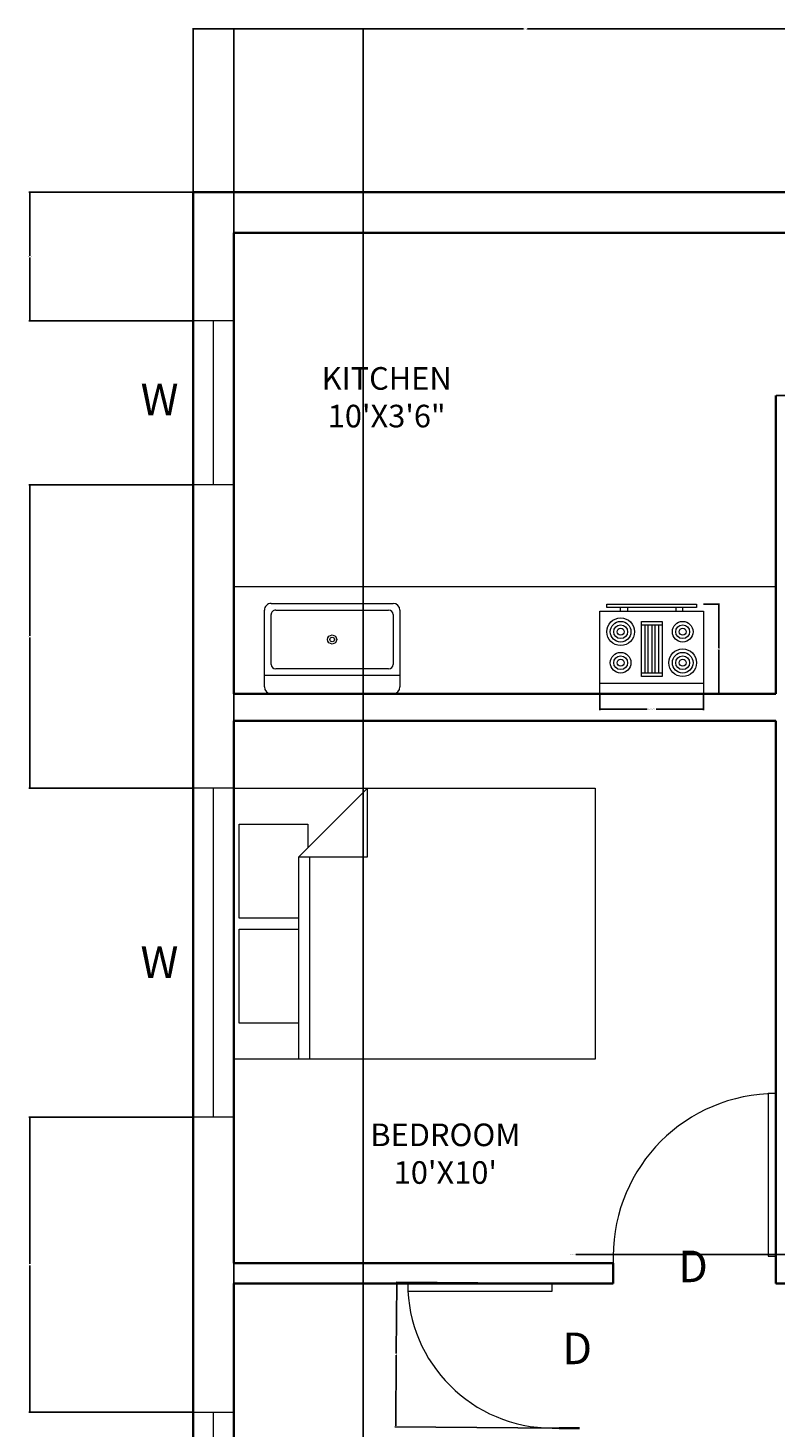
# Model space of a CAD drawing. Units: inches. Extents: x 1939 to 2674, y 558 to 1170.
# Tile 2 of 6: x 1939 to 2104, y 861 to 1170. Entities that reach past the tile are written whole.
import ezdxf

# ---------------------------------------------------------------- set-up
doc = ezdxf.new("R2010")
doc.units = ezdxf.units.IN
for name, color, linetype, lineweight in [('A-ANNO-DIMS', 2, 'Continuous', 18), ('A-ANNO-TEXT', 7, 'Continuous', 18), ('A-AREA-IDEN', 7, 'Continuous', 18), ('A-DOOR', 3, 'Continuous', 18), ('A-EQPM', 8, 'Continuous', 18), ('A-FLOR-CASE', 8, 'Continuous', 18), ('A-FLOR-FIXT', 9, 'Continuous', 18), ('A-FURN', 8, 'Continuous', 13), ('A-GLAZ', 4, 'Continuous', 18), ('A-WALL', 7, 'Continuous', 35)]:
    doc.layers.add(name, color=color, linetype=linetype, lineweight=lineweight)
doc.styles.get("Standard").update_dxf_attribs({"font": 'arial.ttf'})
doc.dimstyles.get("Standard").update_dxf_attribs({"dimtxt": 0.18, "dimasz": 0.18, "dimexe": 0.18, "dimexo": 0.0625, "dimgap": 0.09, "dimtad": 0, "dimtih": 1, "dimtoh": 1, "dimdec": 4, "dimzin": 0, "dimdsep": 46, "dimtxsty": 'Standard', "dimcen": 0.09, "dimadec": 0, "dimazin": 0, "dimtfac": 1, "dimtdec": 4, "dimtofl": 0, "dimtmove": 0, "dimatfit": 3, "dimfxl": 1, "dimtolj": 1, "dimtzin": 0, "dimarcsym": 0})

# ---------------------------------------------------------------- blocks, each defined once
blk = doc.blocks.new('Bed - Queen')
for p, q in [((0, -80.00003), (0, 0)), ((0, 0), (59.99999, 0)), ((59.99999, 0), (59.99999, -80.00003)), ((7.99999, -1.2), (28.79998, -1.2)), ((7.99999, -14.4), (7.99999, -1.2)), ((28.79998, -1.2), (28.79998, -14.4)), ((31.19999, -1.2), (51.99999, -1.2)), ((31.19999, -14.4), (31.19999, -1.2)), ((51.99999, -1.2), (51.99999, -16.4)), ((0, -14.4), (44.8, -14.4)), ((59.99999, -29.6), (44.8, -14.4)), ((44.8, -14.4), (44.8, -29.6)), ((44.8, -16.8), (0, -16.8)), ((51.99999, -16.4), (46.79936, -16.4)), ((44.8, -29.6), (59.99999, -29.6)), ((59.99999, -80.00003), (0, -80.00003))]:
    blk.add_line(p, q)
blk = doc.blocks.new('Sink-single - 30 in top')
blk.add_line((-15, -3.999996), (15, -3.999996))
for points in [[(-13.5, 0), (13.5, 0)], [(-15, -18.499996), (-15, -1.5)], [(15, -1.5), (15, -18.499996)], [(-12.5, -5.499996), (12.5, -5.499996)], [(-13.5, -17.499996), (-13.5, -6.499996)], [(13.5, -6.499996), (13.5, -17.499996)], [(12.5, -18.499996), (-12.5, -18.499996)], [(13.5, -19.999996), (-13.5, -19.999996)]]:
    blk.add_lwpolyline(points)
for radius in [1, 0.5]:
    blk.add_circle((0, -11.999996), radius)
for centre, radius, start, end in [((-13.5, -1.5), 1.5, 90, 180), ((13.5, -1.5), 1.5, 0, 90), ((-12.5, -6.499996), 1, 90, 180), ((12.5, -6.499996), 1, 0, 90), ((-13.5, -18.499996), 1.5, 180, 270), ((-12.5, -17.499996), 1, 180, 270), ((12.5, -17.499996), 1, 270, 0), ((13.5, -18.499996), 1.5, 270, 0)]:
    blk.add_arc(centre, radius, start, end)
blk = doc.blocks.new('Range-Oven - 30 in top')
for p, q in [((0, -3), (30, -3)), ((12, -6), (18, -6)), ((13, -20), (13, -6)), ((14, -6), (14, -20)), ((15, -20), (15, -6)), ((16, -6), (16, -20)), ((17, -20), (17, -6)), ((18, -20), (12, -20)), ((6, -24), (6, -25)), ((8, -25), (8, -24)), ((22, -25), (22, -24)), ((24, -24), (24, -25))]:
    blk.add_line(p, q)
for points in [[(0, -24), (0, 0), (30, 0), (30, -24)], [(12, -21), (12, -5), (18, -5), (18, -21)], [(2, -26), (2, -25), (28, -25), (28, -26)]]:
    blk.add_lwpolyline(points, close=True)
for centre, radius in [((6, -9), 4), ((6, -9), 3), ((6, -9), 2), ((6, -9), 1), ((24, -9), 3), ((24, -9), 2), ((24, -9), 1), ((6, -18), 3), ((6, -18), 2), ((24, -18), 4), ((24, -18), 3), ((24, -18), 2), ((6, -18), 1), ((24, -18), 1)]:
    blk.add_circle(centre, radius)
blk = doc.blocks.new('*U10')
for p, q in [((0, 0), (0, -6)), ((-36, 0), (-36, -6))]:
    blk.add_line(p, q)
blk.add_lwpolyline([(0, 0), (0, 36), (-1.75, 36), (-1.75, 0)], close=True)
blk.add_arc((0, 0), 36, 90, 180)
blk = doc.blocks.new('*U12')
for p, q in [((0, 0), (0, -6)), ((-32, 0), (-32, -6))]:
    blk.add_line(p, q)
blk.add_lwpolyline([(0, 0), (0, 32), (-1.75, 32), (-1.75, 0)], close=True)
blk.add_arc((0, 0), 32, 90, 180)
blk = doc.blocks.new('WIN-KITCHEN')
for p, q in [((9, 36.3), (0, 36.3)), ((4.5, 0), (4.5, 36.3)), ((9, 0), (0, 0))]:
    blk.add_line(p, q)
blk = doc.blocks.new('WIN-BEDROOM')
for p, q in [((9, 72.81), (0, 72.81)), ((4.5, 0), (4.5, 72.81)), ((9, 0), (0, 0))]:
    blk.add_line(p, q)
blk = doc.blocks.new('VENT-TOILET')
for p, q in [((0, 41.35), (9, 41.35)), ((4.5, 0), (4.5, 41.35)), ((0, 0), (9, 0))]:
    blk.add_line(p, q)
blk = doc.blocks.new('*D32')
at = {"layer": 'A-ANNO-DIMS', "color": 0, "lineweight": -2, "transparency": 16777216}
for p, q in [((2065.1, 1023.05), (2065.1, 1019.5)), ((2087.97, 1023.05), (2087.97, 1019.5)), ((2065.28, 1019.68), (2075.53, 1019.68)), ((2087.79, 1019.68), (2077.54, 1019.68))]:
    blk.add_line(p, q, dxfattribs=at)
at = {"layer": 'A-ANNO-DIMS', "color": 0, "transparency": 16777216}
for points in [[(2065.28, 1019.71), (2065.28, 1019.65), (2065.1, 1019.68)], [(2087.79, 1019.71), (2087.79, 1019.65), (2087.97, 1019.68)]]:
    blk.add_solid(points, dxfattribs=at)
at = {"layer": 'Defpoints', "color": 0, "transparency": 16777216}
for p in [(2065.1, 1023.11), (2087.97, 1023.11), (2065.1, 1019.68)]:
    blk.add_point(p, dxfattribs=at)
at = {"layer": 'A-ANNO-DIMS', "color": 0, "transparency": 16777216, "insert": (2076.54, 1019.68), "char_height": 0.18, "attachment_point": 5}
blk.add_mtext('\\A1;RANGE 23 TYP.', dxfattribs=at)
blk = doc.blocks.new('*D33')
at = {"layer": 'A-ANNO-DIMS', "color": 0, "lineweight": -2, "transparency": 16777216}
for p, q in [((2088.03, 1042.93), (2091.58, 1042.93)), ((2091.4, 1042.75), (2091.4, 1033.2)), ((2091.4, 1023.29), (2091.4, 1032.84)), ((2088.03, 1023.11), (2091.58, 1023.11))]:
    blk.add_line(p, q, dxfattribs=at)
at = {"layer": 'A-ANNO-DIMS', "color": 0, "transparency": 16777216}
for points in [[(2091.37, 1042.75), (2091.43, 1042.75), (2091.4, 1042.93)], [(2091.37, 1023.29), (2091.43, 1023.29), (2091.4, 1023.11)]]:
    blk.add_solid(points, dxfattribs=at)
at = {"layer": 'Defpoints', "color": 0, "transparency": 16777216}
for p in [(2087.97, 1042.93), (2087.97, 1023.11), (2091.4, 1023.11)]:
    blk.add_point(p, dxfattribs=at)
at = {"layer": 'A-ANNO-DIMS', "color": 0, "transparency": 16777216, "insert": (2091.4, 1033.02), "char_height": 0.18, "attachment_point": 5}
blk.add_mtext('\\A1;20 TYP.', dxfattribs=at)
blk = doc.blocks.new('*D55')
at = {"layer": 'A-ANNO-DIMS', "color": 0, "lineweight": -2, "transparency": 16777216}
for p, q in [((2056.24, 892.61), (2019.97, 892.89)), ((2020.15, 892.71), (2020.03, 877.07)), ((2019.9, 861.07), (2020.02, 876.71)), ((2055.99, 860.61), (2019.72, 860.89))]:
    blk.add_line(p, q, dxfattribs=at)
at = {"layer": 'A-ANNO-DIMS', "color": 0, "transparency": 16777216}
for points in [[(2020.12, 892.71), (2020.18, 892.71), (2020.15, 892.89)], [(2019.87, 861.07), (2019.93, 861.07), (2019.9, 860.89)]]:
    blk.add_solid(points, dxfattribs=at)
at = {"layer": 'Defpoints', "color": 0, "transparency": 16777216}
for p in [(2020.15, 892.89), (2056.3, 892.61), (2056.05, 860.61)]:
    blk.add_point(p, dxfattribs=at)
at = {"layer": 'A-ANNO-DIMS', "color": 0, "transparency": 16777216, "insert": (2020.02, 876.89), "char_height": 0.18, "attachment_point": 5}
blk.add_mtext('\\A1;32', dxfattribs=at)
blk = doc.blocks.new('*D59')
at = {"layer": 'A-ANNO-DIMS', "color": 0, "lineweight": -2, "transparency": 16777216}
for p, q in [((1975.05, 1134.17), (1975.05, 1170.44)), ((1975.23, 1170.26), (2048.18, 1170.26)), ((2122.04, 1170.26), (2049.09, 1170.26)), ((2122.22, 1134.17), (2122.22, 1170.44))]:
    blk.add_line(p, q, dxfattribs=at)
at = {"layer": 'A-ANNO-DIMS', "color": 0, "transparency": 16777216}
for points in [[(1975.23, 1170.29), (1975.23, 1170.23), (1975.05, 1170.26)], [(2122.04, 1170.29), (2122.04, 1170.23), (2122.22, 1170.26)]]:
    blk.add_solid(points, dxfattribs=at)
at = {"layer": 'Defpoints', "color": 0, "transparency": 16777216}
for p in [(2122.22, 1170.26), (1975.05, 1134.11), (2122.22, 1134.11)]:
    blk.add_point(p, dxfattribs=at)
at = {"layer": 'A-ANNO-DIMS', "color": 0, "transparency": 16777216, "insert": (2048.64, 1170.26), "char_height": 0.18, "attachment_point": 5}
blk.add_mtext('\\A1;147.18', dxfattribs=at)
blk = doc.blocks.new('*D61')
at = {"layer": 'A-ANNO-DIMS', "color": 0, "lineweight": -2, "transparency": 16777216}
for p, q in [((1984.05, 603.17), (1984.05, 1170.44)), ((1984.23, 1170.26), (1997.89, 1170.26)), ((2012.48, 1170.26), (1998.82, 1170.26)), ((2012.66, 603.17), (2012.66, 1170.44))]:
    blk.add_line(p, q, dxfattribs=at)
at = {"layer": 'A-ANNO-DIMS', "color": 0, "transparency": 16777216}
for points in [[(1984.23, 1170.29), (1984.23, 1170.23), (1984.05, 1170.26)], [(2012.48, 1170.29), (2012.48, 1170.23), (2012.66, 1170.26)]]:
    blk.add_solid(points, dxfattribs=at)
at = {"layer": 'Defpoints', "color": 0, "transparency": 16777216}
for p in [(2012.66, 1170.26), (1984.05, 603.11), (2012.66, 603.11)]:
    blk.add_point(p, dxfattribs=at)
at = {"layer": 'A-ANNO-DIMS', "color": 0, "transparency": 16777216, "insert": (1998.36, 1170.26), "char_height": 0.18, "attachment_point": 5}
blk.add_mtext('\\A1;28.616', dxfattribs=at)
blk = doc.blocks.new('*D62')
at = {"layer": 'A-ANNO-DIMS', "color": 0, "lineweight": -2, "transparency": 16777216}
for p, q in [((1974.99, 1134.11), (1938.72, 1134.11)), ((1938.9, 1133.93), (1938.9, 1120.04)), ((1938.9, 1105.78), (1938.9, 1119.67)), ((1974.99, 1105.6), (1938.72, 1105.6))]:
    blk.add_line(p, q, dxfattribs=at)
at = {"layer": 'A-ANNO-DIMS', "color": 0, "transparency": 16777216}
for points in [[(1938.87, 1133.93), (1938.93, 1133.93), (1938.9, 1134.11)], [(1938.87, 1105.78), (1938.93, 1105.78), (1938.9, 1105.6)]]:
    blk.add_solid(points, dxfattribs=at)
at = {"layer": 'Defpoints', "color": 0, "transparency": 16777216}
for p in [(1975.05, 1134.11), (1938.9, 1105.6), (1975.05, 1105.6)]:
    blk.add_point(p, dxfattribs=at)
at = {"layer": 'A-ANNO-DIMS', "color": 0, "transparency": 16777216, "insert": (1938.9, 1119.86), "char_height": 0.18, "attachment_point": 5}
blk.add_mtext('\\A1;28.507', dxfattribs=at)
blk = doc.blocks.new('*D63')
at = {"layer": 'A-ANNO-DIMS', "color": 0, "lineweight": -2, "transparency": 16777216}
for p, q in [((1974.99, 1069.31), (1938.72, 1069.31)), ((1938.9, 1069.13), (1938.9, 1035.95)), ((1938.9, 1002.4), (1938.9, 1035.58)), ((1974.99, 1002.22), (1938.72, 1002.22))]:
    blk.add_line(p, q, dxfattribs=at)
at = {"layer": 'A-ANNO-DIMS', "color": 0, "transparency": 16777216}
for points in [[(1938.87, 1069.13), (1938.93, 1069.13), (1938.9, 1069.31)], [(1938.87, 1002.4), (1938.93, 1002.4), (1938.9, 1002.22)]]:
    blk.add_solid(points, dxfattribs=at)
at = {"layer": 'Defpoints', "color": 0, "transparency": 16777216}
for p in [(1975.05, 1069.31), (1938.9, 1002.22), (1975.05, 1002.22)]:
    blk.add_point(p, dxfattribs=at)
at = {"layer": 'A-ANNO-DIMS', "color": 0, "transparency": 16777216, "insert": (1938.9, 1035.76), "char_height": 0.18, "attachment_point": 5}
blk.add_mtext('\\A1;67.09', dxfattribs=at)
blk = doc.blocks.new('*D64')
at = {"layer": 'A-ANNO-DIMS', "color": 0, "lineweight": -2, "transparency": 16777216}
for p, q in [((1974.99, 929.41), (1938.72, 929.41)), ((1938.9, 929.23), (1938.9, 896.94)), ((1938.9, 864.29), (1938.9, 896.58)), ((1974.99, 864.11), (1938.72, 864.11))]:
    blk.add_line(p, q, dxfattribs=at)
at = {"layer": 'A-ANNO-DIMS', "color": 0, "transparency": 16777216}
for points in [[(1938.87, 929.23), (1938.93, 929.23), (1938.9, 929.41)], [(1938.87, 864.29), (1938.93, 864.29), (1938.9, 864.11)]]:
    blk.add_solid(points, dxfattribs=at)
at = {"layer": 'Defpoints', "color": 0, "transparency": 16777216}
for p in [(1975.05, 929.41), (1938.9, 864.11), (1975.05, 864.11)]:
    blk.add_point(p, dxfattribs=at)
at = {"layer": 'A-ANNO-DIMS', "color": 0, "transparency": 16777216, "insert": (1938.9, 896.76), "char_height": 0.18, "attachment_point": 5}
blk.add_mtext('\\A1;65.3', dxfattribs=at)
blk = doc.blocks.new('*D65')
at = {"layer": 'A-ANNO-DIMS', "color": 0, "lineweight": -2, "transparency": 16777216}
for p, q in [((2122.29, 1125.11), (2674.38, 1125.11)), ((2674.2, 1124.93), (2674.2, 1107.29)), ((2674.2, 1089.29), (2674.2, 1106.93)), ((2104.11, 1089.11), (2674.38, 1089.11))]:
    blk.add_line(p, q, dxfattribs=at)
at = {"layer": 'A-ANNO-DIMS', "color": 0, "transparency": 16777216}
for points in [[(2674.17, 1124.93), (2674.23, 1124.93), (2674.2, 1125.11)], [(2674.17, 1089.29), (2674.23, 1089.29), (2674.2, 1089.11)]]:
    blk.add_solid(points, dxfattribs=at)
at = {"layer": 'Defpoints', "color": 0, "transparency": 16777216}
for p in [(2122.22, 1125.11), (2674.2, 1125.11), (2104.05, 1089.11)]:
    blk.add_point(p, dxfattribs=at)
at = {"layer": 'A-ANNO-DIMS', "color": 0, "transparency": 16777216, "insert": (2674.2, 1107.11), "char_height": 0.18, "attachment_point": 5}
blk.add_mtext('\\A1;36', dxfattribs=at)
blk = doc.blocks.new('*D73')
at = {"layer": 'A-ANNO-DIMS', "color": 0, "lineweight": -2, "transparency": 16777216}
for p, q in [((2061.53, 899.04), (2133.39, 899.04)), ((2254.68, 899.04), (2254.86, 899.04)), ((2254.77, 898.95), (2254.77, 899.13))]:
    blk.add_line(p, q, dxfattribs=at)
at = {"layer": 'A-ANNO-DIMS', "color": 0, "transparency": 16777216}
blk.add_solid([(2133.39, 899.07), (2133.39, 899.01), (2133.57, 899.04)], dxfattribs=at)
at = {"layer": 'Defpoints', "color": 0, "transparency": 16777216}
for p in [(2133.57, 899.04), (2254.77, 899.04)]:
    blk.add_point(p, dxfattribs=at)
at = {"layer": 'A-ANNO-DIMS', "color": 0, "transparency": 16777216, "insert": (2060.85, 899.04), "char_height": 0.18, "attachment_point": 5}
blk.add_mtext('\\A1;2X R121.2', dxfattribs=at)
blk = doc.blocks.new('*D74')
at = {"layer": 'A-ANNO-DIMS', "color": 0, "lineweight": -2, "transparency": 16777216}
for p, q in [((2059.77, 899.04), (2127.39, 899.04)), ((2241.73, 899.04), (2241.91, 899.04)), ((2241.82, 898.95), (2241.82, 899.13))]:
    blk.add_line(p, q, dxfattribs=at)
at = {"layer": 'A-ANNO-DIMS', "color": 0, "transparency": 16777216}
blk.add_solid([(2127.39, 899.07), (2127.39, 899.01), (2127.57, 899.04)], dxfattribs=at)
at = {"layer": 'Defpoints', "color": 0, "transparency": 16777216}
for p in [(2127.57, 899.04), (2241.82, 899.04)]:
    blk.add_point(p, dxfattribs=at)
at = {"layer": 'A-ANNO-DIMS', "color": 0, "transparency": 16777216, "insert": (2059.02, 899.04), "char_height": 0.18, "attachment_point": 5}
blk.add_mtext('\\A1;2X R114.25', dxfattribs=at)

msp = doc.modelspace()

# ---------------------------------------------------------------- linework, layer by layer
at = {"layer": 'A-FLOR-CASE'}
msp.add_line((1984.0479, 1046.8584), (2104.048, 1046.8584), dxfattribs=at)
at = {"layer": 'A-WALL'}
for p, q in [((2638.048, 1134.1102), (1975.0479, 1134.1102)), ((1975.0479, 1134.1102), (1975.0479, 594.1102)), ((1984.0479, 1125.1102), (1984.0479, 1023.1102)), ((1984.0479, 1125.1102), (2230.048, 1125.1102)), ((2104.048, 1089.1102), (2104.048, 1023.1102)), ((2104.048, 1023.1102), (1984.0479, 1023.1102)), ((1984.0479, 1017.1102), (1984.0479, 897.1102)), ((2104.048, 1017.1102), (1984.0479, 1017.1102)), ((2104.048, 1017.1102), (2104.048, 897.1102)), ((2068.048, 897.1102), (1984.0479, 897.1102)), ((2068.048, 897.1102), (2068.048, 892.6102)), ((2104.048, 897.1102), (2104.048, 892.6102)), ((2068.048, 892.6102), (1984.0479, 892.6102)), ((1984.0479, 892.6102), (1984.0479, 775.6102)), ((2110.048, 892.6102), (2104.048, 892.6102)), ((2060.548, 860.6102), (2056.048, 860.6102))]:
    msp.add_line(p, q, dxfattribs=at)

# ---------------------------------------------------------------- block references
at = {"layer": 'A-DOOR'}
msp.add_blockref('*U10', (2104.048, 898.6102), dxfattribs=at)
at = {"layer": 'A-DOOR', "rotation": 90}
msp.add_blockref('*U12', (2054.548, 892.6102), dxfattribs=at)
at = {"layer": 'A-EQPM', "xscale": 0.762387585591576, "yscale": 0.762387585591576, "zscale": 0.762387585591576, "rotation": 180}
msp.add_blockref('Range-Oven - 30 in top', (2087.971, 1023.1102), dxfattribs=at)
at = {"layer": 'A-FLOR-FIXT', "rotation": 180}
msp.add_blockref('Sink-single - 30 in top', (2005.8303, 1023.1102), dxfattribs=at)
at = {"layer": 'A-FURN', "rotation": 90}
msp.add_blockref('Bed - Queen', (1984.0479, 942.2222), dxfattribs=at)
at = {"layer": 'A-GLAZ'}
for name, p in [('WIN-KITCHEN', (1975.0479, 1069.3076)), ('WIN-BEDROOM', (1975.0479, 929.4108)), ('VENT-TOILET', (1975.0479, 822.7612))]:
    msp.add_blockref(name, p, dxfattribs=at)

# ---------------------------------------------------------------- texts
at = {"layer": 'A-ANNO-TEXT', "char_height": 7, "attachment_point": 1}
for s, insert in [('\\pxqc;W', (1956.6898, 1091.745)), ('\\pxqc;W', (1956.6616, 967.1949)), ('\\pxqc;D', (2074.7399, 899.8795)), ('\\pxqc;D', (2049.1137, 881.735))]:
    msp.add_mtext_dynamic_manual_height_columns(s, width=21.893501, gutter_width=12.5, heights=[0], dxfattribs=dict(at, insert=insert))
at = {"layer": 'A-AREA-IDEN', "char_height": 5, "attachment_point": 1}
for s, insert in [('\\pxqc;KITCHEN\\P10\'X3\'6"', (1998.3374, 1095.3899)), ("\\pxqc;BEDROOM\\P10'X10'", (2011.3206, 927.9875))]:
    msp.add_mtext_dynamic_manual_height_columns(s, width=39.116177, gutter_width=12.5, heights=[0], dxfattribs=dict(at, insert=insert))

# ---------------------------------------------------------------- dimensions: what is measured, and where the dimension line sits
at = {"layer": 'A-ANNO-DIMS'}
for base, p1, p2, override, picture, middle in [((2122.2249, 1170.2602), (1975.0479, 1134.1102), (2122.2249, 1134.1102), {"dimdec": 2, "dimlfac": 1, "dimrnd": 0, "dimzin": 0, "dimdsep": 46, "dimlunit": 2}, '*D59', (2048.6364, 1170.2602)), ((2012.6641, 1170.2602), (1984.0479, 603.1102), (2012.6641, 603.1102), {"dimdec": 3, "dimlfac": 1, "dimrnd": 0, "dimzin": 0, "dimdsep": 46, "dimlunit": 2}, '*D61', (1998.356, 1170.2602))]:
    dim = msp.add_linear_dim(base=base, p1=p1, p2=p2, dimstyle='Standard', override=override, dxfattribs=at)
    dim.commit()
    dim.dimension.update_dxf_attribs({"geometry": picture, "text_midpoint": middle})
for base, p1, p2, angle, override, picture, middle in [((1938.898, 1105.6031), (1975.0479, 1134.1102), (1975.0479, 1105.6031), 90, {"dimdec": 3, "dimlfac": 1, "dimrnd": 0, "dimzin": 0, "dimdsep": 46, "dimlunit": 2}, '*D62', (1938.898, 1119.8567)), ((2674.198, 1125.1102), (2104.048, 1089.1102), (2122.2249, 1125.1102), 90, {"dimdec": 0, "dimlfac": 1, "dimrnd": 0, "dimzin": 0, "dimdsep": 46, "dimlunit": 2}, '*D65', (2674.198, 1107.1102)), ((1938.898, 1002.2222), (1975.0479, 1069.3076), (1975.0479, 1002.2222), 90, {"dimdec": 2, "dimlfac": 1, "dimrnd": 0, "dimzin": 0, "dimdsep": 46, "dimlunit": 2}, '*D63', (1938.898, 1035.7649)), ((1938.898, 864.1102), (1975.0479, 929.4108), (1975.0479, 864.1102), 90, {"dimdec": 1, "dimlfac": 1, "dimrnd": 0, "dimzin": 0, "dimdsep": 46, "dimlunit": 2}, '*D64', (1938.898, 896.7605)), ((2020.1491, 892.8926), (2056.048, 860.6102), (2056.298, 892.6102), 89.552386, {"dimdec": 0, "dimlfac": 1, "dimrnd": 0, "dimzin": 0, "dimdsep": 46, "dimlunit": 2}, '*D55', (2020.0241, 876.8926))]:
    dim = msp.add_linear_dim(base=base, p1=p1, p2=p2, angle=angle, dimstyle='Standard', override=override, dxfattribs=at)
    dim.commit()
    dim.dimension.update_dxf_attribs({"geometry": picture, "text_midpoint": middle})
for base, p1, p2, angle, text, picture, middle in [((2091.4017, 1023.1102), (2087.971, 1042.9323), (2087.971, 1023.1102), 270, '<> TYP.', '*D33', (2091.4017, 1033.0212)), ((2065.0994, 1019.6795), (2087.971, 1023.1102), (2065.0994, 1023.1102), 180, 'RANGE <> TYP.', '*D32', (2076.5352, 1019.6795))]:
    dim = msp.add_linear_dim(base=base, p1=p1, p2=p2, angle=angle, text=text, dimstyle='Standard', override={"dimdec": 0, "dimlfac": 1, "dimrnd": 0, "dimzin": 0, "dimdsep": 46, "dimlunit": 2}, dxfattribs=at)
    dim.commit()
    dim.dimension.update_dxf_attribs({"geometry": picture, "text_midpoint": middle})
for center, mpoint, override, picture, middle in [((2241.8209, 899.043), (2127.5709, 899.043), {"dimdec": 2, "dimlfac": 1, "dimrnd": 0, "dimzin": 0, "dimdsep": 46, "dimlunit": 2}, '*D74', (2059.0209, 899.043)), ((2254.7677, 899.043), (2133.5709, 899.043), {"dimdec": 1, "dimlfac": 1, "dimrnd": 0, "dimzin": 0, "dimdsep": 46, "dimlunit": 2}, '*D73', (2060.8528, 899.043))]:
    dim = msp.add_radius_dim(center=center, mpoint=mpoint, text='2X <>', dimstyle='Standard', override=override, dxfattribs=at)
    dim.commit()
    dim.dimension.update_dxf_attribs({"geometry": picture, "text_midpoint": middle, "dimtype": 164})

doc.saveas('drawing.dxf')
